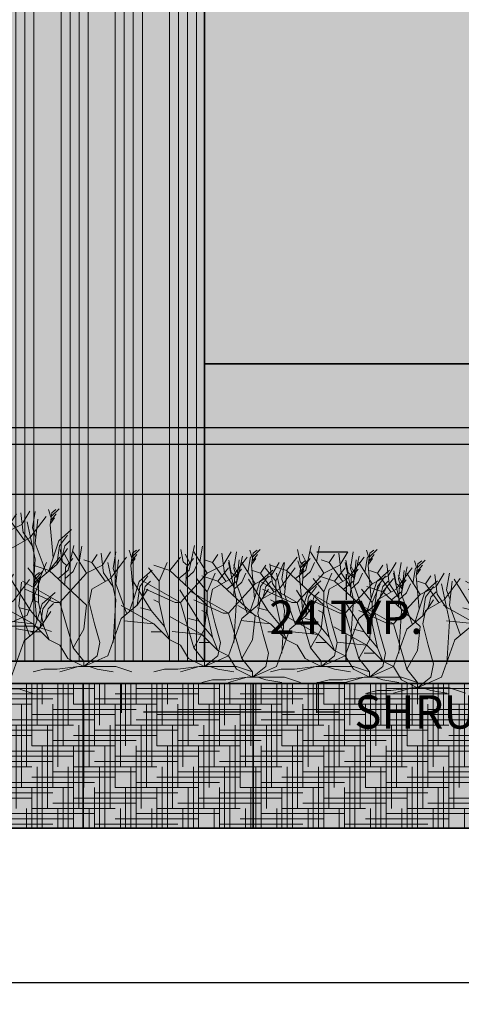
# Model space of a CAD drawing. Units: inches. Extents: x 221 to 874, y 171 to 738.
# Tile 2 of 11: x 373 to 452, y 171 to 348. Entities that reach past the tile are written whole.
import ezdxf

# ---------------------------------------------------------------- set-up
doc = ezdxf.new("R2010")
doc.units = ezdxf.units.IN
doc.header["$MEASUREMENT"] = 0
for name, color, linetype, lineweight in [('A-ANNO-DIMS', 2, 'Continuous', 18), ('A-ELEV', 7, 'Continuous', 35), ('A-ELEV-PATT', 8, 'Continuous', 13), ('L-PLNT', 3, 'Continuous', 13)]:
    doc.layers.add(name, color=color, linetype=linetype, lineweight=lineweight)
doc.styles.get("Standard").update_dxf_attribs({"font": 'arial.ttf'})
doc.dimstyles.get("Standard").update_dxf_attribs({"dimtxt": 6, "dimasz": 4, "dimexe": 0.18, "dimexo": 0.0625, "dimgap": 0.09, "dimtad": 0, "dimtih": 1, "dimtoh": 1, "dimdec": 0, "dimzin": 0, "dimdsep": 46, "dimlunit": 3, "dimtxsty": 'Standard', "dimcen": 0.09, "dimadec": 0, "dimazin": 0, "dimtfac": 1, "dimtdec": 0, "dimtofl": 0, "dimtmove": 0, "dimatfit": 3, "dimfxl": 1, "dimtolj": 1, "dimtzin": 0, "dimarcsym": 0})

# ---------------------------------------------------------------- blocks, each defined once
blk = doc.blocks.new('SHRUB-A')
for p, q in [((15.5, 17.76), (13.1, 21.6)), ((18.38, 19.2), (19.82, 21.6)), ((6.86, 16.32), (8.3, 19.68)), ((8.78, 18.24), (10.7, 20.64)), ((19.82, 16.8), (22.7, 20.64)), ((6.86, 16.32), (4.94, 18.72)), ((8.78, 18.24), (5.9, 19.2)), ((15.5, 12), (8.78, 18.24)), ((10.7, 12.48), (15.5, 17.76)), ((15.5, 17.76), (18.38, 19.2)), ((5.42, 11.04), (1.91, 16.66)), ((10.7, 12.48), (3.98, 16.32)), ((6.86, 12.48), (6.86, 16.32)), ((16.46, 14.88), (19.82, 16.8)), ((25.1, 15.36), (26.54, 17.28)), ((9.74, 12.48), (4.46, 14.88)), ((15.98, 12.48), (16.46, 14.88)), ((24.62, 12), (25.1, 15.36)), ((24.62, 12), (26.54, 14.88)), ((6.86, 12.48), (5.9, 12.96)), ((7.82, 8.16), (6.86, 12.48)), ((10.7, 12.48), (9.74, 12.48)), ((13.1, 4.32), (10.7, 12.48)), ((16.94, 8.64), (15.98, 12.48)), ((5.9, 8.64), (0, 11.96)), ((5.42, 11.04), (3.5, 11.52)), ((7.82, 8.16), (5.42, 11.04)), ((15.02, 7.68), (15.5, 12)), ((21.74, 9.6), (24.62, 12)), ((5.9, 8.64), (0.53, 9.22)), ((19.34, 2.88), (21.74, 9.6)), ((8.78, 5.76), (5.9, 8.64)), ((8.78, 5.76), (7.82, 8.16)), ((13.1, 4.32), (15.02, 7.68)), ((17.9, 5.28), (16.94, 8.64)), ((10.7, 4.8), (8.78, 5.76)), ((12.14, 2.4), (10.7, 4.8)), ((15.02, 1.92), (13.1, 4.32)), ((17.42, 2.88), (17.9, 5.28)), ((15.02, 0.96), (12.14, 2.4)), ((15.02, 0.96), (19.34, 2.88)), ((15.02, 0.96), (17.42, 2.88)), ((15.02, 0.96), (15.02, 1.92)), ((15.02, 0.96), (20.78, 0.96)), ((20.78, 0.96), (23.66, 0))]:
    blk.add_line(p, q)
blk = doc.blocks.new('GRASS-TUFT')
for p, q in [((0.58, 10.54), (1.31, 11.09)), ((0.28, 8.35), (0.58, 10.54)), ((0.83, 2.4), (0.28, 8.35)), ((1.8, 5.45), (4.12, 7.49)), ((0.83, 2.4), (1.8, 5.45)), ((0, 0), (0.83, 2.4))]:
    blk.add_line(p, q)
blk = doc.blocks.new('GRASS-SPRIG')
for p, q in [((1.44, 3.36), (0, 3.84)), ((1.44, 3.36), (2.4, 4.8)), ((3.84, 0), (1.44, 3.36))]:
    blk.add_line(p, q)
blk = doc.blocks.new('SHRUB-C')
for p, q in [((15.5, 19.68), (13.1, 23.52)), ((18.38, 21.12), (19.82, 23.52)), ((6.86, 18.24), (8.3, 21.6)), ((8.78, 20.16), (10.7, 22.56)), ((19.82, 18.72), (22.7, 22.56)), ((24.14, 17.76), (21.74, 21.6)), ((27.02, 19.2), (28.46, 21.6)), ((6.86, 18.24), (4.94, 20.64)), ((8.78, 20.16), (5.9, 21.12)), ((15.5, 13.92), (8.78, 20.16)), ((10.7, 14.4), (15.5, 19.68)), ((15.5, 19.68), (18.38, 21.12)), ((15.5, 16.32), (16.94, 19.68)), ((17.42, 18.24), (19.34, 20.64)), ((28.46, 16.8), (31.34, 20.64)), ((5.42, 12.96), (1.91, 18.58)), ((10.7, 14.4), (3.98, 18.24)), ((6.86, 14.4), (6.86, 18.24)), ((15.5, 16.32), (13.58, 18.72)), ((17.42, 18.24), (14.54, 19.2)), ((16.46, 16.8), (19.82, 18.72)), ((24.14, 12), (17.42, 18.24)), ((19.34, 12.48), (24.14, 17.76)), ((24.14, 17.76), (27.02, 19.2)), ((25.1, 17.28), (26.54, 19.2)), ((9.74, 14.4), (4.46, 16.8)), ((14.06, 11.04), (10.55, 16.66)), ((19.34, 12.48), (12.62, 16.32)), ((15.5, 12.48), (15.5, 16.32)), ((15.98, 14.4), (16.46, 16.8)), ((24.62, 13.92), (25.1, 17.28)), ((24.62, 13.92), (26.54, 16.8)), ((25.1, 14.88), (28.46, 16.8)), ((33.74, 15.36), (35.18, 17.28)), ((6.86, 14.4), (5.9, 14.88)), ((7.82, 10.08), (6.86, 14.4)), ((10.7, 14.4), (9.74, 14.4)), ((13.1, 6.24), (10.7, 14.4)), ((18.38, 12.48), (13.1, 14.88)), ((16.94, 10.56), (15.98, 14.4)), ((24.62, 12.48), (25.1, 14.88)), ((33.26, 12), (33.74, 15.36)), ((33.26, 12), (35.18, 14.88)), ((5.9, 10.56), (0, 13.88)), ((5.42, 12.96), (3.5, 13.44)), ((7.82, 10.08), (5.42, 12.96)), ((15.5, 12.48), (14.54, 12.96)), ((15.02, 9.6), (15.5, 13.92)), ((16.46, 8.16), (15.5, 12.48)), ((19.34, 12.48), (18.38, 12.48)), ((21.74, 4.32), (19.34, 12.48)), ((21.74, 11.52), (24.62, 13.92)), ((25.58, 8.64), (24.62, 12.48)), ((5.9, 10.56), (0.53, 11.14)), ((14.54, 8.64), (8.64, 11.96)), ((14.06, 11.04), (12.14, 11.52)), ((16.46, 8.16), (14.06, 11.04)), ((19.34, 4.8), (21.74, 11.52)), ((23.66, 7.68), (24.14, 12)), ((30.38, 9.6), (33.26, 12)), ((8.78, 7.68), (5.9, 10.56)), ((8.78, 7.68), (7.82, 10.08)), ((14.54, 8.64), (9.17, 9.22)), ((13.1, 6.24), (15.02, 9.6)), ((17.9, 7.2), (16.94, 10.56)), ((27.98, 2.88), (30.38, 9.6)), ((10.7, 6.72), (8.78, 7.68)), ((17.42, 5.76), (14.54, 8.64)), ((17.42, 5.76), (16.46, 8.16)), ((17.42, 4.8), (17.9, 7.2)), ((21.74, 4.32), (23.66, 7.68)), ((26.54, 5.28), (25.58, 8.64)), ((12.14, 4.32), (10.7, 6.72)), ((15.02, 3.84), (13.1, 6.24)), ((19.34, 4.8), (17.42, 5.76)), ((15.02, 2.88), (12.14, 4.32)), ((15.02, 2.88), (19.34, 4.8)), ((15.02, 2.88), (17.42, 4.8)), ((15.02, 2.88), (15.02, 3.84)), ((20.78, 2.4), (19.34, 4.8)), ((23.66, 1.92), (21.74, 4.32)), ((26.06, 2.88), (26.54, 5.28)), ((15.02, 2.88), (20.78, 2.88)), ((20.78, 2.88), (23.66, 1.92)), ((23.66, 0.96), (20.78, 2.4)), ((23.66, 0.96), (27.98, 2.88)), ((23.66, 0.96), (26.06, 2.88)), ((23.66, 0.96), (23.66, 1.92)), ((23.66, 0.96), (29.42, 0.96)), ((29.42, 0.96), (32.3, 0))]:
    blk.add_line(p, q)
blk = doc.blocks.new('*D18')
at = {"layer": 'A-ANNO-DIMS', "color": 0, "lineweight": -2, "transparency": 16777216}
for p, q in [((391.06, 228.81), (391.06, 223.42)), ((426.24, 228.81), (426.24, 223.42)), ((395.06, 223.6), (422.24, 223.6)), ((426.24, 223.6), (430.24, 223.6))]:
    blk.add_line(p, q, dxfattribs=at)
at = {"layer": 'A-ANNO-DIMS', "color": 0, "transparency": 16777216}
for points in [[(395.06, 224.27), (395.06, 222.93), (391.06, 223.6)], [(422.24, 224.27), (422.24, 222.93), (426.24, 223.6)]]:
    blk.add_solid(points, dxfattribs=at)
at = {"layer": 'Defpoints', "color": 0, "transparency": 16777216}
for p in [(391.06, 228.88), (426.24, 228.88), (426.24, 223.6)]:
    blk.add_point(p, dxfattribs=at)
at = {"layer": 'A-ANNO-DIMS', "color": 0, "transparency": 16777216, "insert": (464.94, 223.6), "char_height": 6, "attachment_point": 5}
blk.add_mtext('\\A1;SHRUB C 35 TYP.', dxfattribs=at)
blk = doc.blocks.new('*D19')
at = {"layer": 'A-ANNO-DIMS', "color": 0, "lineweight": -2, "transparency": 16777216}
for p, q in [((426.3, 252.4), (431.7, 252.4)), ((431.52, 248.4), (431.52, 243.74)), ((431.52, 232.88), (431.52, 237.53)), ((426.3, 228.88), (431.7, 228.88))]:
    blk.add_line(p, q, dxfattribs=at)
at = {"layer": 'A-ANNO-DIMS', "color": 0, "transparency": 16777216}
for points in [[(430.85, 248.4), (432.18, 248.4), (431.52, 252.4)], [(430.85, 232.88), (432.18, 232.88), (431.52, 228.88)]]:
    blk.add_solid(points, dxfattribs=at)
at = {"layer": 'Defpoints', "color": 0, "transparency": 16777216}
for p in [(426.24, 252.4), (431.52, 252.4), (426.24, 228.88)]:
    blk.add_point(p, dxfattribs=at)
at = {"layer": 'A-ANNO-DIMS', "color": 0, "transparency": 16777216, "insert": (431.52, 240.64), "char_height": 6, "attachment_point": 5}
blk.add_mtext('\\A1;24 TYP.', dxfattribs=at)
blk = doc.blocks.new('*D20')
at = {"layer": 'A-ANNO-DIMS', "color": 0, "lineweight": -2, "transparency": 16777216}
for p, q in [((313.08, 202.65), (313.08, 174.79)), ((805.08, 202.65), (805.08, 174.79)), ((317.08, 174.97), (552.27, 174.97)), ((801.08, 174.97), (565.89, 174.97))]:
    blk.add_line(p, q, dxfattribs=at)
at = {"layer": 'A-ANNO-DIMS', "color": 0, "transparency": 16777216}
for points in [[(317.08, 175.63), (317.08, 174.3), (313.08, 174.97)], [(801.08, 175.63), (801.08, 174.3), (805.08, 174.97)]]:
    blk.add_solid(points, dxfattribs=at)
at = {"layer": 'Defpoints', "color": 0, "transparency": 16777216}
for p in [(313.08, 202.72), (805.08, 202.72), (805.08, 174.97)]:
    blk.add_point(p, dxfattribs=at)
at = {"layer": 'A-ANNO-DIMS', "color": 0, "transparency": 16777216, "insert": (559.08, 174.97), "char_height": 6, "attachment_point": 5}
blk.add_mtext('\\A1;492', dxfattribs=at)
blk = doc.blocks.new('*D67')
at = {"layer": 'A-ANNO-DIMS', "color": 0, "lineweight": -2, "transparency": 16777216}
for p, q in [((231.54, 271.72), (231.54, 275.72)), ((231.54, 275.72), (235.54, 275.72)), ((541.02, 271.72), (231.36, 271.72)), ((231.54, 266.72), (231.54, 267.72)), ((541.02, 262.72), (231.36, 262.72))]:
    blk.add_line(p, q, dxfattribs=at)
at = {"layer": 'A-ANNO-DIMS', "color": 0, "transparency": 16777216}
for points in [[(230.88, 267.72), (232.21, 267.72), (231.54, 271.72)], [(230.88, 266.72), (232.21, 266.72), (231.54, 262.72)]]:
    blk.add_solid(points, dxfattribs=at)
at = {"layer": 'Defpoints', "color": 0, "transparency": 16777216}
for p in [(231.54, 271.72), (541.08, 271.72), (541.08, 262.72)]:
    blk.add_point(p, dxfattribs=at)
at = {"layer": 'A-ANNO-DIMS', "color": 0, "transparency": 16777216, "insert": (237.61, 275.72), "char_height": 6, "attachment_point": 5}
blk.add_mtext('\\A1;9', dxfattribs=at)
blk = doc.blocks.new('*D68')
at = {"layer": 'A-ANNO-DIMS', "color": 0, "lineweight": -2, "transparency": 16777216}
for p, q in [((231.54, 278.72), (231.54, 282.72)), ((231.54, 282.72), (235.54, 282.72)), ((541.02, 274.72), (231.36, 274.72)), ((541.02, 271.72), (231.36, 271.72)), ((231.54, 267.72), (231.54, 263.72))]:
    blk.add_line(p, q, dxfattribs=at)
at = {"layer": 'A-ANNO-DIMS', "color": 0, "transparency": 16777216}
for points in [[(230.88, 278.72), (232.21, 278.72), (231.54, 274.72)], [(230.88, 267.72), (232.21, 267.72), (231.54, 271.72)]]:
    blk.add_solid(points, dxfattribs=at)
at = {"layer": 'Defpoints', "color": 0, "transparency": 16777216}
for p in [(231.54, 274.72), (541.08, 274.72), (541.08, 271.72)]:
    blk.add_point(p, dxfattribs=at)
at = {"layer": 'A-ANNO-DIMS', "color": 0, "transparency": 16777216, "insert": (237.6, 282.72), "char_height": 6, "attachment_point": 5}
blk.add_mtext('\\A1;3', dxfattribs=at)

msp = doc.modelspace()

# ---------------------------------------------------------------- hatches: boundary and pattern name
at = {"layer": 'A-ELEV-PATT'}
h = msp.add_hatch(color=256, dxfattribs=at)
h.dxf.hatch_style = 1
h.paths.add_polyline_path([(349.0786, 286.1996), (313.0786, 286.1996), (313.0786, 232.7164), (349.0786, 232.7164)])
h.paths.add_polyline_path([(464.0786, 286.1996), (406.0786, 286.1996), (406.0786, 232.7164), (464.0786, 232.7164)])
h.paths.add_polyline_path([(541.0786, 286.1996), (493.0786, 286.1996), (493.0786, 232.7164), (541.0786, 232.7164)])
h.paths.add_polyline_path([(541.0786, 370.7164), (493.0786, 370.7164), (493.0786, 286.1996), (541.0786, 286.1996)])
h.paths.add_polyline_path([(464.0786, 370.7164), (406.0786, 370.7164), (406.0786, 286.1996), (464.0786, 286.1996)])
h.paths.add_polyline_path([(349.0786, 370.7164), (313.0786, 370.7164), (313.0786, 286.1996), (349.0786, 286.1996)])
h.paths.add_polyline_path([(349.0786, 454.7164), (313.0786, 454.7164), (313.0786, 370.7164), (349.0786, 370.7164)])
h.paths.add_polyline_path([(464.0786, 454.7164), (406.0786, 454.7164), (406.0786, 370.7164), (464.0786, 370.7164)])
h.paths.add_polyline_path([(541.0786, 418.7164), (541.0786, 454.7164), (493.0786, 454.7164), (493.0786, 370.7164), (541.0786, 370.7164)])
h.paths.add_polyline_path([(541.0786, 550.7164), (493.0786, 550.7164), (493.0786, 454.7164), (541.0786, 454.7164)])
h.paths.add_polyline_path([(464.0786, 550.7164), (406.0786, 550.7164), (406.0786, 454.7164), (464.0786, 454.7164)])
h.paths.add_polyline_path([(349.0786, 550.7164), (313.0786, 550.7164), (313.0786, 454.7164), (349.0786, 454.7164)])
h.paths.add_polyline_path([(349.0786, 586.7164), (313.0786, 586.7164), (313.0786, 550.7164), (349.0786, 550.7164)])
h.paths.add_polyline_path([(464.0786, 586.7164), (406.0786, 586.7164), (406.0786, 550.7164), (464.0786, 550.7164)])
h.paths.add_polyline_path([(541.0786, 574.7164), (541.0786, 586.7164), (493.0786, 586.7164), (493.0786, 550.7164), (541.0786, 550.7164)])
h.paths.add_polyline_path([(541.0786, 670.7164), (493.0786, 670.7164), (493.0786, 586.7164), (541.0786, 586.7164)])
h.paths.add_polyline_path([(464.0786, 670.7164), (406.0786, 670.7164), (406.0786, 586.7164), (464.0786, 586.7164)])
h.paths.add_polyline_path([(349.0786, 670.7164), (313.0786, 670.7164), (313.0786, 586.7164), (349.0786, 586.7164)])
h.paths.add_polyline_path([(406.0786, 706.7164), (313.0786, 706.7164), (313.0786, 670.7164), (349.0786, 670.7164), (406.0786, 670.7164)])
h.paths.add_polyline_path([(464.0786, 706.7164), (406.0786, 706.7164), (406.0786, 670.7164), (464.0786, 670.7164)])
h.paths.add_polyline_path([(541.0786, 706.7164), (493.0786, 706.7164), (493.0786, 688.7164), (493.0786, 670.7164), (541.0786, 670.7164)])
h.paths.add_polyline_path([(660.0786, 610.7164), (541.0786, 610.7164), (541.0786, 586.7164), (541.0786, 574.7164), (660.0786, 574.7164)])
h.paths.add_polyline_path([(781.0786, 610.7164), (660.0786, 610.7164), (660.0786, 574.7164), (769.0786, 574.7164), (781.0786, 574.7164)])
h.paths.add_polyline_path([(781.0786, 574.7164), (769.0786, 574.7164), (769.0786, 476.1199), (781.0786, 476.1199)])
h.paths.add_polyline_path([(781.0786, 476.1199), (769.0786, 476.1199), (769.0786, 457.7164), (781.0786, 457.7164)])
h.paths.add_polyline_path([(781.0786, 377.1023), (705.9097, 377.1023), (705.9097, 286.1996), (781.0786, 286.1996)])
h.paths.add_polyline_path([(741.9618, 338.8486), (756.9618, 338.8486), (756.9618, 329.8486), (741.9618, 329.8486)], flags=16)
h.paths.add_polyline_path([(648.9097, 377.1023), (598.0786, 377.1023), (598.0786, 286.1996), (648.9097, 286.1996)])
h.paths.add_polyline_path([(781.0786, 286.1996), (705.9097, 286.1996), (705.9097, 280.7164), (648.9097, 280.7164), (648.9097, 286.1996), (598.0786, 286.1996), (598.0786, 280.7164), (550.0786, 280.7164), (550.0786, 286.1996), (541.0786, 286.1996), (541.0786, 274.7164), (781.0786, 274.7164)])
h.paths.add_polyline_path([(660.0786, 562.7164), (546.3477, 562.7164), (546.3477, 457.7164), (660.0786, 457.7164)])
h = msp.add_hatch(color=256, dxfattribs=at)
h.paths.add_polyline_path([(406.0786, 670.7164), (349.0786, 670.7164), (349.0786, 454.7164), (406.0786, 454.7164)])
h.paths.add_polyline_path([(406.0786, 454.7164), (349.0786, 454.7164), (349.0786, 232.7164), (406.0786, 232.7164)])
h = msp.add_hatch(dxfattribs=at)
h.set_pattern_fill('ANSI34', color=256, scale=13, angle=45, style=0)
h.paths.add_polyline_path([(406.0786, 670.7164), (349.0786, 670.7164), (349.0786, 454.7164), (406.0786, 454.7164)])
h.paths.add_polyline_path([(406.0786, 454.7164), (349.0786, 454.7164), (349.0786, 232.7164), (406.0786, 232.7164)])
msp.add_hatch(color=256, dxfattribs=at).paths.add_polyline_path([(313.0786, 232.7164), (313.0786, 228.7164), (541.0786, 228.7164), (541.0786, 232.7164)])
h = msp.add_hatch(color=256, dxfattribs=at)
h.set_gradient(color1=(147, 149, 152), color2=(91, 91, 91), name='CURVED')
h.paths.add_polyline_path([(384.2386, 202.7164), (384.2386, 228.7164), (338.5139, 228.7164), (338.5139, 202.7164)])
h = msp.add_hatch(dxfattribs=at)
h.set_pattern_fill('HOUND', color=256, scale=15, style=0)
h.paths.add_polyline_path([(384.2386, 228.7164), (338.5139, 228.7164), (338.5139, 202.7164), (384.2386, 202.7164)])
h = msp.add_hatch(color=256, dxfattribs=at)
h.set_gradient(color1=(99, 100, 102), color2=(91, 91, 91), rotation=180, name='INVCURVED')
h.paths.add_polyline_path([(414.8291, 202.7164), (414.8291, 228.7164), (384.2386, 228.7164), (384.2386, 202.7164)])
h = msp.add_hatch(dxfattribs=at)
h.set_pattern_fill('HOUND', color=256, scale=15, style=0)
h.paths.add_polyline_path([(414.8291, 228.7164), (384.2386, 228.7164), (384.2386, 202.7164), (414.8291, 202.7164)])
h = msp.add_hatch(color=256, dxfattribs=at)
h.set_gradient(color1=(147, 149, 152), color2=(91, 91, 91), name='CURVED')
h.paths.add_polyline_path([(462.8078, 202.7164), (462.8078, 228.7164), (414.8291, 228.7164), (414.8291, 202.7164)])
h = msp.add_hatch(dxfattribs=at)
h.set_pattern_fill('HOUND', color=256, scale=15, style=0)
h.paths.add_polyline_path([(462.8078, 228.7164), (414.8291, 228.7164), (414.8291, 202.7164), (462.8078, 202.7164)])

# ---------------------------------------------------------------- linework, layer by layer
at = {"layer": 'A-ELEV'}
for p, q in [((406.0786, 232.7164), (406.0786, 670.7164)), ((406.0786, 286.1996), (464.0786, 286.1996)), ((541.0786, 232.7164), (313.0786, 232.7164)), ((541.0786, 228.7164), (313.0786, 228.7164)), ((384.2386, 228.7164), (384.2386, 202.7164)), ((414.8291, 228.7164), (414.8291, 202.7164)), ((805.0786, 202.7164), (313.0786, 202.7164))]:
    msp.add_line(p, q, dxfattribs=at)
at = {"layer": 'L-PLNT'}
for p, q in [((373.4238, 255.8394), (372.9968, 259.4384)), ((373.2298, 257.2984), (374.6698, 259.6984)), ((374.6698, 254.8984), (377.5498, 258.7384)), ((375.1328, 256.7004), (375.6218, 259.6734)), ((378.0018, 259.9864), (378.4288, 258.6564)), ((378.4898, 258.1084), (379.4058, 259.2034)), ((378.5508, 258.8124), (379.8938, 260.1424)), ((370.3498, 255.8584), (373.2298, 257.2984)), ((375.6298, 251.0584), (374.1898, 257.7784)), ((375.6298, 253.9384), (376.1098, 258.2584)), ((378.3678, 257.4824), (379.0998, 258.4994)), ((375.1328, 253.4134), (373.4238, 255.9174)), ((375.7438, 254.9004), (375.1328, 256.7004)), ((379.9498, 253.4584), (381.3898, 255.3784)), ((371.3098, 252.9784), (374.6698, 254.8984)), ((377.5498, 248.6584), (375.6298, 253.9384)), ((379.4698, 250.0984), (379.9498, 253.4584)), ((380.4298, 251.5384), (380.9098, 253.4584)), ((380.9098, 253.4584), (381.8698, 254.4184)), ((381.5648, 249.0854), (382.5408, 253.5454)), ((383.5178, 250.5714), (384.0058, 253.3884)), ((403.2856, 249.0854), (404.2616, 253.5454)), ((405.2386, 250.5714), (405.7266, 253.3884)), ((424.2856, 249.0854), (425.2616, 253.5454)), ((426.2386, 250.5714), (426.7266, 253.3884)), ((378.1178, 249.0364), (380.0378, 251.4364)), ((379.4698, 250.0984), (381.3898, 252.9784)), ((380.5268, 250.5714), (380.0998, 252.8404)), ((381.7178, 250.4154), (380.8938, 251.9804)), ((384.8378, 248.5564), (382.4378, 252.3964)), ((387.9118, 248.5374), (387.4848, 252.1364)), ((387.7178, 249.9964), (389.1578, 252.3964)), ((389.1578, 247.5964), (392.0378, 251.4364)), ((389.6208, 249.3984), (390.1098, 252.3714)), ((392.4898, 252.6844), (392.9168, 251.3544)), ((392.9778, 250.8064), (393.8938, 251.9014)), ((393.0388, 251.5104), (394.3818, 252.8404)), ((402.2476, 250.5714), (401.8206, 252.8404)), ((403.4386, 250.4154), (402.6146, 251.9804)), ((409.6326, 248.5374), (409.2056, 252.1364)), ((411.3416, 249.3984), (411.8306, 252.3714)), ((411.9256, 247.1654), (412.9016, 251.6254)), ((413.8786, 248.6514), (414.3666, 251.4684)), ((414.2106, 252.6844), (414.6376, 251.3544)), ((414.5156, 249.9454), (414.8206, 252.1364)), ((414.6986, 250.8064), (415.6146, 251.9014)), ((414.7596, 251.5104), (416.1026, 252.8404)), ((414.8206, 252.1364), (415.5536, 252.6844)), ((420.8386, 249.0364), (422.7586, 251.4364)), ((423.2476, 250.5714), (422.8206, 252.8404)), ((424.4386, 250.4154), (423.6146, 251.9804)), ((427.5586, 248.5564), (425.1586, 252.3964)), ((430.6326, 248.5374), (430.2056, 252.1364)), ((430.4386, 249.9964), (431.8786, 252.3964)), ((431.8786, 247.5964), (434.7586, 251.4364)), ((432.3416, 249.3984), (432.8306, 252.3714)), ((432.9256, 247.1654), (433.9016, 251.6254)), ((434.8786, 248.6514), (435.3666, 251.4684)), ((435.2106, 252.6844), (435.6376, 251.3544)), ((435.6986, 250.8064), (436.6146, 251.9014)), ((435.7596, 251.5104), (437.1026, 252.8404)), ((375.1498, 243.3784), (375.6298, 251.0584)), ((378.1178, 249.0364), (375.2378, 249.9964)), ((376.1978, 247.1164), (377.6378, 250.4764)), ((376.5898, 247.6984), (379.4698, 250.0984)), ((381.3208, 249.8674), (380.5268, 250.5714)), ((381.0768, 249.6324), (382.3578, 251.1974)), ((382.4188, 248.8504), (383.1518, 250.4934)), ((384.8378, 248.5564), (387.7178, 249.9964)), ((390.1178, 243.7564), (388.6778, 250.4764)), ((390.1178, 246.6364), (390.5978, 250.9564)), ((392.8558, 250.1804), (393.5878, 251.1974)), ((403.0416, 249.8674), (402.2476, 250.5714)), ((402.7976, 249.6324), (404.0786, 251.1974)), ((404.1396, 248.8504), (404.8726, 250.4934)), ((411.8386, 243.7564), (410.3986, 250.4764)), ((410.8876, 248.6514), (410.4606, 250.9204)), ((412.0786, 248.4954), (411.2546, 250.0604)), ((411.8386, 246.6364), (412.3186, 250.9564)), ((415.0646, 243.9994), (414.5156, 249.9454)), ((414.5766, 250.1804), (415.3086, 251.1974)), ((418.2726, 246.6174), (417.8456, 250.2164)), ((420.8386, 249.0364), (417.9586, 249.9964)), ((418.9186, 247.1164), (420.3586, 250.4764)), ((419.9816, 247.4784), (420.4706, 250.4514)), ((422.8506, 250.7644), (423.2776, 249.4344)), ((424.0416, 249.8674), (423.2476, 250.5714)), ((423.3386, 248.8864), (424.2546, 249.9814)), ((423.3996, 249.5904), (424.7426, 250.9204)), ((423.7976, 249.6324), (425.0786, 251.1974)), ((425.1396, 248.8504), (425.8726, 250.4934)), ((427.5586, 248.5564), (430.4386, 249.9964)), ((432.8386, 243.7564), (431.3986, 250.4764)), ((431.8876, 248.6514), (431.4606, 250.9204)), ((433.0786, 248.4954), (432.2546, 250.0604)), ((432.8386, 246.6364), (433.3186, 250.9564)), ((436.1986, 246.6364), (433.7986, 250.4764)), ((435.5766, 250.1804), (436.3086, 251.1974)), ((439.2726, 246.6174), (438.8456, 250.2164)), ((439.0786, 248.0764), (440.5186, 250.4764)), ((440.9816, 247.4784), (441.4706, 250.4514)), ((441.5656, 245.2454), (442.5416, 249.7054)), ((443.8506, 250.7644), (444.2776, 249.4344)), ((444.3386, 248.8864), (445.2546, 249.9814)), ((444.3996, 249.5904), (445.7426, 250.9204)), ((376.1978, 247.1164), (374.2778, 249.5164)), ((375.0498, 248.6844), (375.4768, 247.3544)), ((375.5378, 246.8064), (376.4538, 247.9014)), ((375.5988, 247.5104), (376.9418, 248.8404)), ((384.8378, 242.7964), (378.1178, 249.0364)), ((379.6728, 247.5204), (381.5648, 249.0854)), ((380.0378, 243.2764), (384.8378, 248.5564)), ((380.9548, 246.4244), (381.0768, 249.6324)), ((381.0158, 247.5984), (382.4188, 248.8504)), ((389.6208, 246.1114), (387.9118, 248.6154)), ((390.2318, 247.5984), (389.6208, 249.3984)), ((394.4378, 246.1564), (395.8778, 248.0764)), ((401.3936, 247.5204), (403.2856, 249.0854)), ((402.6756, 246.4244), (402.7976, 249.6324)), ((402.7366, 247.5984), (404.1396, 248.8504)), ((411.3416, 246.1114), (409.6326, 248.6154)), ((411.6816, 247.9474), (410.8876, 248.6514)), ((411.9526, 247.5984), (411.3416, 249.3984)), ((411.4376, 247.7124), (412.7186, 249.2774)), ((412.7796, 246.9304), (413.5126, 248.5734)), ((416.0416, 247.0504), (418.3606, 249.0854)), ((418.9186, 247.1164), (416.9986, 249.5164)), ((420.4786, 241.8364), (419.0386, 248.5564)), ((420.4786, 244.7164), (420.9586, 249.0364)), ((427.5586, 242.7964), (420.8386, 249.0364)), ((422.3936, 247.5204), (424.2856, 249.0854)), ((422.7586, 243.2764), (427.5586, 248.5564)), ((423.2166, 248.2604), (423.9486, 249.2774)), ((423.6756, 246.4244), (423.7976, 249.6324)), ((423.7366, 247.5984), (425.1396, 248.8504)), ((429.4786, 247.1164), (426.5986, 248.0764)), ((427.5586, 245.1964), (428.9986, 248.5564)), ((429.4786, 247.1164), (431.3986, 249.5164)), ((432.3416, 246.1114), (430.6326, 248.6154)), ((432.6816, 247.9474), (431.8876, 248.6514)), ((432.9526, 247.5984), (432.3416, 249.3984)), ((432.4376, 247.7124), (433.7186, 249.2774)), ((433.7796, 246.9304), (434.5126, 248.5734)), ((436.1986, 246.6364), (439.0786, 248.0764)), ((437.1586, 246.1564), (438.5986, 248.0764)), ((441.4786, 241.8364), (440.0386, 248.5564)), ((440.5276, 246.7314), (440.1006, 249.0004)), ((440.5186, 245.6764), (443.3986, 249.5164)), ((441.7186, 246.5754), (440.8946, 248.1404)), ((441.4786, 244.7164), (441.9586, 249.0364)), ((444.8386, 244.7164), (442.4386, 248.5564)), ((443.5186, 246.7314), (444.0066, 249.5484)), ((444.2166, 248.2604), (444.9486, 249.2774)), ((447.9126, 244.6974), (447.4856, 248.2964)), ((447.7186, 246.1564), (449.1586, 248.5564)), ((449.6216, 245.5584), (450.1106, 248.5314)), ((374.7578, 241.8364), (371.2428, 247.4514)), ((372.6778, 242.6364), (373.1578, 246.9564)), ((380.0378, 243.2764), (373.3178, 247.1164)), ((374.1898, 240.9784), (376.5898, 247.6984)), ((375.4158, 246.1804), (376.1478, 247.1974)), ((376.1978, 243.2764), (376.1978, 247.1164)), ((385.7978, 245.6764), (389.1578, 247.5964)), ((392.0378, 241.3564), (390.1178, 246.6364)), ((393.9578, 242.7964), (394.4378, 246.1564)), ((394.9178, 244.2364), (395.3978, 246.1564)), ((395.3978, 246.1564), (396.3578, 247.1164)), ((410.0336, 245.6004), (411.9256, 247.1654)), ((411.3156, 244.5044), (411.4376, 247.7124)), ((411.3766, 245.6784), (412.7796, 246.9304)), ((413.7586, 241.3564), (411.8386, 246.6364)), ((417.4786, 241.8364), (413.9636, 247.4514)), ((415.0646, 243.9994), (416.0416, 247.0504)), ((422.7586, 243.2764), (416.0386, 247.1164)), ((416.6386, 244.2364), (417.1186, 246.1564)), ((417.1186, 246.1564), (418.0786, 247.1164)), ((419.9816, 244.1914), (418.2726, 246.6954)), ((418.9186, 243.2764), (418.9186, 247.1164)), ((420.5926, 245.6784), (419.9816, 247.4784)), ((427.5586, 245.1964), (425.6386, 247.5964)), ((428.5186, 245.6764), (431.8786, 247.5964)), ((436.1986, 240.8764), (429.4786, 247.1164)), ((431.0336, 245.6004), (432.9256, 247.1654)), ((431.3986, 241.3564), (436.1986, 246.6364)), ((432.3156, 244.5044), (432.4376, 247.7124)), ((432.3766, 245.6784), (433.7796, 246.9304)), ((434.7586, 241.3564), (432.8386, 246.6364)), ((438.1186, 245.1964), (435.2386, 246.1564)), ((436.1986, 243.2764), (437.6386, 246.6364)), ((436.6786, 242.7964), (437.1586, 246.1564)), ((437.6386, 244.2364), (438.1186, 246.1564)), ((438.1186, 245.1964), (440.0386, 247.5964)), ((438.1186, 246.1564), (439.0786, 247.1164)), ((440.9816, 244.1914), (439.2726, 246.6954)), ((441.3216, 246.0274), (440.5276, 246.7314)), ((441.5926, 245.6784), (440.9816, 247.4784)), ((441.0776, 245.7924), (442.3586, 247.3574)), ((442.4196, 245.0104), (443.1526, 246.6534)), ((444.8386, 244.7164), (447.7186, 246.1564)), ((445.7986, 244.2364), (447.2386, 246.1564)), ((450.1186, 239.9164), (448.6786, 246.6364)), ((449.1586, 243.7564), (452.0386, 247.5964)), ((450.1186, 242.7964), (450.5986, 247.1164)), ((379.0778, 243.2764), (373.7978, 245.6764)), ((385.3178, 243.2764), (385.7978, 245.6764)), ((393.9578, 242.7964), (395.8778, 245.6764)), ((421.7986, 243.2764), (416.5186, 245.6764)), ((422.3986, 239.4364), (420.4786, 244.7164)), ((426.1186, 239.9164), (422.6036, 245.5314)), ((431.3986, 241.3564), (424.6786, 245.1964)), ((425.7586, 244.2364), (426.7186, 245.1964)), ((427.5586, 241.3564), (427.5586, 245.1964)), ((428.0386, 243.2764), (428.5186, 245.6764)), ((436.1986, 243.2764), (434.2786, 245.6764)), ((436.6786, 242.7964), (438.5986, 245.6764)), ((437.1586, 243.7564), (440.5186, 245.6764)), ((444.8386, 238.9564), (438.1186, 245.1964)), ((439.6736, 243.6804), (441.5656, 245.2454)), ((440.0386, 239.4364), (444.8386, 244.7164)), ((440.9556, 242.5844), (441.0776, 245.7924)), ((441.0166, 243.7584), (442.4196, 245.0104)), ((443.3986, 239.4364), (441.4786, 244.7164)), ((446.7586, 244.2364), (447.7186, 245.1964)), ((449.6216, 242.2714), (447.9126, 244.7754)), ((450.2326, 243.7584), (449.6216, 245.5584)), ((375.2378, 239.4364), (369.3348, 242.7574)), ((374.5978, 237.3564), (372.6778, 242.6364)), ((376.1978, 243.2764), (375.2378, 243.7564)), ((377.1578, 238.9564), (376.1978, 243.2764)), ((377.9578, 242.1564), (378.9178, 243.1164)), ((380.0378, 243.2764), (379.0778, 243.2764)), ((382.4378, 235.1164), (380.0378, 243.2764)), ((384.3578, 238.4764), (384.8378, 242.7964)), ((386.2778, 239.4364), (385.3178, 243.2764)), ((389.6378, 236.0764), (390.1178, 243.7564)), ((391.0778, 240.3964), (393.9578, 242.7964)), ((411.3586, 236.0764), (411.8386, 243.7564)), ((417.9586, 239.4364), (412.0556, 242.7574)), ((414.2386, 241.5964), (415.0646, 243.9994)), ((418.9186, 243.2764), (417.9586, 243.7564)), ((419.8786, 238.9564), (418.9186, 243.2764)), ((422.7586, 243.2764), (421.7986, 243.2764)), ((425.1586, 235.1164), (422.7586, 243.2764)), ((430.4386, 241.3564), (425.1586, 243.7564)), ((425.2786, 242.3164), (425.7586, 244.2364)), ((427.0786, 238.4764), (427.5586, 242.7964)), ((428.9986, 239.4364), (428.0386, 243.2764)), ((434.7586, 237.9964), (431.2436, 243.6114)), ((432.3586, 236.0764), (432.8386, 243.7564)), ((440.0386, 239.4364), (433.3186, 243.2764)), ((433.7986, 240.3964), (436.6786, 242.7964)), ((436.1986, 239.4364), (436.1986, 243.2764)), ((436.6786, 241.3564), (437.1586, 243.7564)), ((445.3186, 240.8764), (445.7986, 244.2364)), ((445.3186, 240.8764), (447.2386, 243.7564)), ((445.7986, 241.8364), (449.1586, 243.7564)), ((446.2786, 242.3164), (446.7586, 244.2364)), ((452.0386, 237.5164), (450.1186, 242.7964)), ((369.8698, 239.0584), (374.1898, 240.9784)), ((374.7578, 241.8364), (372.8378, 242.3164)), ((377.1578, 238.9564), (374.7578, 241.8364)), ((377.4778, 240.2364), (377.9578, 242.1564)), ((417.4786, 241.8364), (415.5586, 242.3164)), ((419.8786, 238.9564), (417.4786, 241.8364)), ((419.9986, 234.1564), (420.4786, 241.8364)), ((426.5986, 237.5164), (420.6956, 240.8374)), ((427.5586, 241.3564), (426.5986, 241.8364)), ((428.5186, 237.0364), (427.5586, 241.3564)), ((431.3986, 241.3564), (430.4386, 241.3564)), ((433.7986, 233.1964), (431.3986, 241.3564)), ((439.0786, 239.4364), (433.7986, 241.8364)), ((435.7186, 236.5564), (436.1986, 240.8764)), ((437.6386, 237.5164), (436.6786, 241.3564)), ((440.9986, 234.1564), (441.4786, 241.8364)), ((442.4386, 238.4764), (445.3186, 240.8764)), ((445.3186, 239.4364), (445.7986, 241.8364)), ((375.2378, 239.4364), (369.8698, 240.0184)), ((369.8698, 239.0584), (375.6298, 239.0584)), ((378.1178, 236.5564), (375.2378, 239.4364)), ((375.6298, 239.0584), (378.5098, 238.0984)), ((387.2378, 236.0764), (386.2778, 239.4364)), ((388.6778, 233.6764), (391.0778, 240.3964)), ((417.9586, 239.4364), (412.5906, 240.0184)), ((420.8386, 236.5564), (417.9586, 239.4364)), ((426.1186, 239.9164), (424.1986, 240.3964)), ((428.5186, 237.0364), (426.1186, 239.9164)), ((429.9586, 236.0764), (428.9986, 239.4364)), ((431.3986, 233.6764), (433.7986, 240.3964)), ((436.1986, 239.4364), (435.2386, 239.9164)), ((437.1586, 235.1164), (436.1986, 239.4364)), ((440.0386, 239.4364), (439.0786, 239.4364)), ((442.4386, 231.2764), (440.0386, 239.4364)), ((446.2786, 235.5964), (445.3186, 239.4364)), ((449.6386, 232.2364), (450.1186, 239.9164)), ((372.2698, 238.5784), (375.1498, 238.0984)), ((376.6778, 237.9964), (374.7578, 237.9964)), ((378.1178, 236.5564), (377.1578, 238.9564)), ((382.4378, 235.1164), (384.3578, 238.4764)), ((398.3986, 237.9964), (396.4786, 237.9964)), ((419.3986, 237.9964), (417.4786, 237.9964)), ((420.8386, 236.5564), (419.8786, 238.9564)), ((426.5986, 237.5164), (421.2306, 238.0984)), ((425.1586, 235.1164), (427.0786, 238.4764)), ((429.4786, 234.6364), (426.5986, 237.5164)), ((435.2386, 235.5964), (429.3356, 238.9174)), ((434.7586, 237.9964), (432.8386, 238.4764)), ((437.1586, 235.1164), (434.7586, 237.9964)), ((438.5986, 234.1564), (437.6386, 237.5164)), ((440.0386, 231.7564), (442.4386, 238.4764)), ((444.3586, 234.6364), (444.8386, 238.9564)), ((451.0786, 236.5564), (453.9586, 238.9564)), ((380.0378, 235.5964), (378.1178, 236.5564)), ((381.4778, 233.1964), (380.0378, 235.5964)), ((386.7578, 233.6764), (387.2378, 236.0764)), ((407.0386, 236.0764), (405.1186, 236.0764)), ((422.7586, 235.5964), (420.8386, 236.5564)), ((424.1986, 233.1964), (422.7586, 235.5964)), ((428.0386, 236.0764), (426.1186, 236.0764)), ((429.4786, 234.6364), (428.5186, 237.0364)), ((429.4786, 233.6764), (429.9586, 236.0764)), ((435.2386, 235.5964), (429.8706, 236.1784)), ((433.7986, 233.1964), (435.7186, 236.5564)), ((438.1186, 232.7164), (435.2386, 235.5964)), ((447.2386, 232.2364), (446.2786, 235.5964)), ((448.6786, 229.8364), (451.0786, 236.5564)), ((384.3578, 232.7164), (382.4378, 235.1164)), ((427.0786, 232.7164), (425.1586, 235.1164)), ((431.3986, 233.6764), (429.4786, 234.6364)), ((436.6786, 234.1564), (434.7586, 234.1564)), ((438.1186, 232.7164), (437.1586, 235.1164)), ((438.1186, 231.7564), (438.5986, 234.1564)), ((442.4386, 231.2764), (444.3586, 234.6364)), ((384.3578, 231.7564), (381.4778, 233.1964)), ((384.3578, 231.7564), (388.6778, 233.6764)), ((384.3578, 231.7564), (386.7578, 233.6764)), ((384.3578, 231.7564), (384.3578, 232.7164)), ((427.0786, 231.7564), (424.1986, 233.1964)), ((427.0786, 231.7564), (431.3986, 233.6764)), ((427.0786, 231.7564), (429.4786, 233.6764)), ((427.0786, 231.7564), (427.0786, 232.7164)), ((432.8386, 231.2764), (431.3986, 233.6764)), ((435.7186, 230.7964), (433.7986, 233.1964)), ((440.0386, 231.7564), (438.1186, 232.7164)), ((446.7586, 229.8364), (447.2386, 232.2364)), ((377.1578, 231.2764), (375.2378, 230.7964)), ((379.5578, 231.2764), (377.1578, 231.2764)), ((383.3978, 231.7564), (379.5578, 231.2764)), ((383.3978, 231.7564), (380.0378, 230.7964)), ((383.3978, 231.7564), (385.3178, 231.7564)), ((384.3578, 231.7564), (390.1178, 231.7564)), ((385.3178, 231.7564), (386.7578, 231.2764)), ((386.7578, 231.2764), (389.6378, 230.7964)), ((390.1178, 231.7564), (392.9978, 230.7964)), ((398.8786, 231.2764), (396.9586, 230.7964)), ((401.2786, 231.2764), (398.8786, 231.2764)), ((405.1186, 231.7564), (401.2786, 231.2764)), ((405.1186, 231.7564), (401.7586, 230.7964)), ((405.1186, 231.7564), (407.0386, 231.7564)), ((407.0386, 231.7564), (408.4786, 231.2764)), ((408.4786, 231.2764), (411.3586, 230.7964)), ((419.8786, 231.2764), (417.9586, 230.7964)), ((422.2786, 231.2764), (419.8786, 231.2764)), ((426.1186, 231.7564), (422.2786, 231.2764)), ((426.1186, 231.7564), (422.7586, 230.7964)), ((426.1186, 231.7564), (428.0386, 231.7564)), ((427.0786, 231.7564), (432.8386, 231.7564)), ((428.0386, 231.7564), (429.4786, 231.2764)), ((429.4786, 231.2764), (432.3586, 230.7964)), ((432.8386, 231.7564), (435.7186, 230.7964)), ((435.7186, 229.8364), (432.8386, 231.2764)), ((435.7186, 229.8364), (440.0386, 231.7564)), ((435.7186, 229.8364), (438.1186, 231.7564)), ((435.7186, 229.8364), (435.7186, 230.7964)), ((441.4786, 229.3564), (440.0386, 231.7564)), ((444.3586, 228.8764), (442.4386, 231.2764)), ((407.5186, 229.3564), (405.5986, 228.8764)), ((409.9186, 229.3564), (407.5186, 229.3564)), ((413.7586, 229.8364), (409.9186, 229.3564)), ((413.7586, 229.8364), (410.3986, 228.8764)), ((413.7586, 229.8364), (415.6786, 229.8364)), ((415.6786, 229.8364), (417.1186, 229.3564)), ((417.1186, 229.3564), (419.9986, 228.8764)), ((428.5186, 229.3564), (426.5986, 228.8764)), ((430.9186, 229.3564), (428.5186, 229.3564)), ((434.7586, 229.8364), (430.9186, 229.3564)), ((434.7586, 229.8364), (431.3986, 228.8764)), ((434.7586, 229.8364), (436.6786, 229.8364)), ((435.7186, 229.8364), (441.4786, 229.8364)), ((436.6786, 229.8364), (438.1186, 229.3564)), ((438.1186, 229.3564), (440.9986, 228.8764)), ((441.4786, 229.8364), (444.3586, 228.8764)), ((444.3586, 227.9164), (441.4786, 229.3564)), ((444.3586, 227.9164), (448.6786, 229.8364)), ((444.3586, 227.9164), (446.7586, 229.8364)), ((444.3586, 227.9164), (444.3586, 228.8764)), ((437.1586, 227.4364), (435.2386, 226.9564)), ((439.5586, 227.4364), (437.1586, 227.4364)), ((443.3986, 227.9164), (439.5586, 227.4364)), ((443.3986, 227.9164), (440.0386, 226.9564)), ((443.3986, 227.9164), (445.3186, 227.9164)), ((444.3586, 227.9164), (450.1186, 227.9164)), ((445.3186, 227.9164), (446.7586, 227.4364)), ((446.7586, 227.4364), (449.6386, 226.9564)), ((450.1186, 227.9164), (452.9986, 226.9564))]:
    msp.add_line(p, q, dxfattribs=at)

# ---------------------------------------------------------------- block references
for name, p in [('GRASS-SPRIG', (369.8702, 254.418)), ('GRASS-TUFT', (378.0302, 248.898)), ('GRASS-SPRIG', (384.3582, 247.116)), ('SHRUB-C', (391.056, 228.876)), ('GRASS-TUFT', (392.5182, 241.596)), ('GRASS-SPRIG', (406.079, 247.116)), ('GRASS-SPRIG', (427.079, 247.116)), ('GRASS-TUFT', (435.239, 241.596)), ('SHRUB-C', (449.056, 228.876)), ('GRASS-SPRIG', (414.719, 245.196)), ('GRASS-TUFT', (422.879, 239.676)), ('GRASS-SPRIG', (435.719, 245.196)), ('GRASS-TUFT', (443.879, 239.676)), ('SHRUB-A', (351.895, 226.796)), ('GRASS-TUFT', (375.0782, 237.596)), ('GRASS-SPRIG', (444.359, 243.276))]:
    msp.add_blockref(name, p, dxfattribs=at)

# ---------------------------------------------------------------- dimensions: what is measured, and where the dimension line sits
at = {"layer": 'A-ANNO-DIMS'}
for base, p1, p2, picture, middle in [((231.5426, 274.7164), (541.0786, 271.7164), (541.0786, 274.7164), '*D68', (237.5972, 282.7164)), ((231.5426, 271.7164), (541.0786, 262.7164), (541.0786, 271.7164), '*D67', (237.6053, 275.7164))]:
    dim = msp.add_linear_dim(base=base, p1=p1, p2=p2, angle=90, dimstyle='Standard', override={"dimdec": 0, "dimlfac": 1, "dimrnd": 0, "dimzin": 0, "dimdsep": 46, "dimlunit": 2}, dxfattribs=at)
    dim.commit()
    dim.dimension.update_dxf_attribs({"geometry": picture, "text_midpoint": middle})
dim = msp.add_linear_dim(base=(431.516, 252.3964), p1=(426.2386, 228.8764), p2=(426.2386, 252.3964), angle=90, text='<> TYP.', dimstyle='Standard', override={"dimdec": 0, "dimrnd": 0, "dimzin": 0, "dimlunit": 2}, dxfattribs=at)
dim.commit()
dim.dimension.update_dxf_attribs({"geometry": '*D19', "text_midpoint": (431.516, 240.6364)})
dim = msp.add_linear_dim(base=(426.2386, 223.5989), p1=(391.0556, 228.8764), p2=(426.2386, 228.8764), text='SHRUB C <> TYP.', dimstyle='Standard', override={"dimdec": 0, "dimrnd": 0, "dimzin": 0, "dimlunit": 2}, dxfattribs=at)
dim.commit()
dim.dimension.update_dxf_attribs({"geometry": '*D18', "text_midpoint": (464.9432, 223.5989)})
dim = msp.add_linear_dim(base=(805.0786, 174.9664), p1=(313.0786, 202.7164), p2=(805.0786, 202.7164), dimstyle='Standard', override={"dimdec": 0, "dimlfac": 1, "dimrnd": 0, "dimzin": 0, "dimdsep": 46, "dimlunit": 2}, dxfattribs=at)
dim.commit()
dim.dimension.update_dxf_attribs({"geometry": '*D20', "text_midpoint": (559.0786, 174.9664)})

doc.saveas('drawing.dxf')
